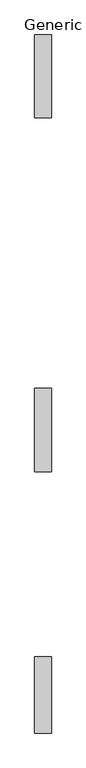
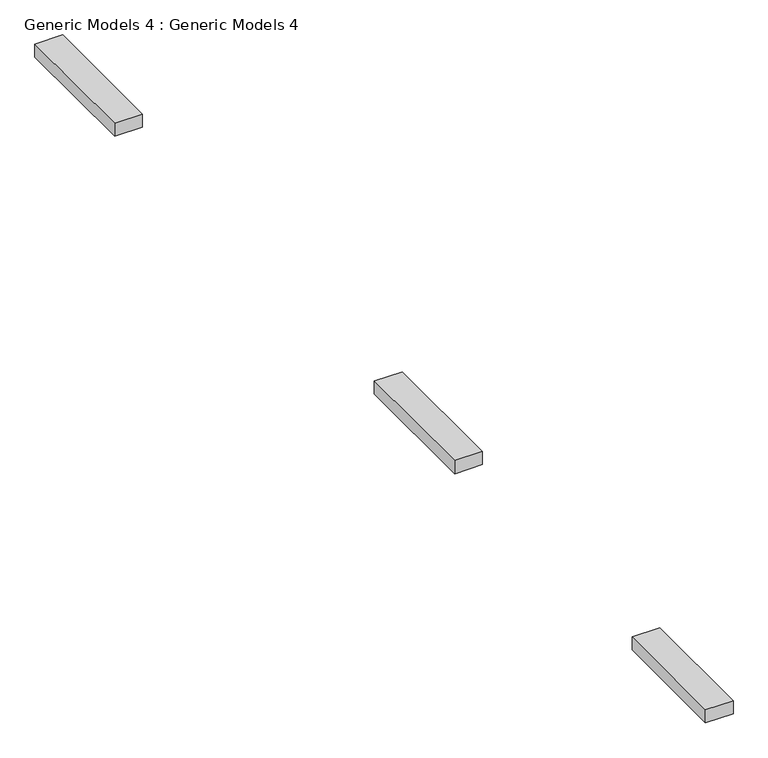
"""IFC4 building model written with IfcOpenShell, lengths in millimetres: proxy geometry, Generic Models 4 : Generic Models 4."""

from ifc_helpers import new_model, si_unit, frame, origin, place, context, project, spatial, polyline, outline, extrude, source, transform, mapped, element, save


def generic_models_4_generic_models_4_21550f0b(model_context):
    return source(origin(), model_context, "Body", "SweptSolid", [
        extrude(outline(polyline([(-15928.6646954, 5920.6374503), (-15928.6646954, 7440.5252636), (-15623.8646954, 7440.5252636), (-15623.8646954, 5920.6374503), (-15928.6646954, 5920.6374503)])), frame((0.0, 0.0, 2260.6), z_axis=(0.0, 0.0, 1.0), x_axis=(1.0, 0.0, 0.0)), (0.0, 0.0, 1.0), 152.4),
        extrude(outline(polyline([(-15928.6646954, -570.5858218), (-15928.6646954, 958.8860888), (-15623.8646954, 958.8860888), (-15623.8646954, -570.5858218), (-15928.6646954, -570.5858218)])), frame((0.0, 0.0, 2260.6), z_axis=(0.0, 0.0, 1.0), x_axis=(1.0, 0.0, 0.0)), (0.0, 0.0, 1.0), 152.4),
        extrude(outline(polyline([(-15928.6646954, -5360.1770128), (-15928.6646954, -3959.3561253), (-15623.8646954, -3959.3561253), (-15623.8646954, -5360.1770128), (-15928.6646954, -5360.1770128)])), frame((0.0, 0.0, 2260.6), z_axis=(0.0, 0.0, 1.0), x_axis=(1.0, 0.0, 0.0)), (0.0, 0.0, 1.0), 152.4),
    ])


if __name__ == "__main__":
    model = new_model("IFC4")
    model_context = context("Model", 3, world=origin())
    ifc_project = project(units=[si_unit("LENGTHUNIT", "METRE", prefix="MILLI")], contexts=[model_context])
    site = spatial("IfcSite", under=ifc_project)
    building = spatial("IfcBuilding", under=site)
    placement = place(None, origin())
    generic_models_4_generic_models_4_shape = generic_models_4_generic_models_4_21550f0b(model_context)
    element("IfcBuildingElementProxy", 1, Name="Generic Models 4 : Generic Models 4", ObjectType="Generic Models 4 : Generic Models 4", at=placement, inside=building, context=model_context, shape_type="MappedRepresentation", body=[
        mapped(generic_models_4_generic_models_4_shape, transform((0.0, 0.0, 0.0), x_axis=(1.0, 0.0, 0.0), y_axis=(0.0, 1.0, 0.0), z_axis=(0.0, 0.0, 1.0))),
    ])
    save(model, "model.ifc")
